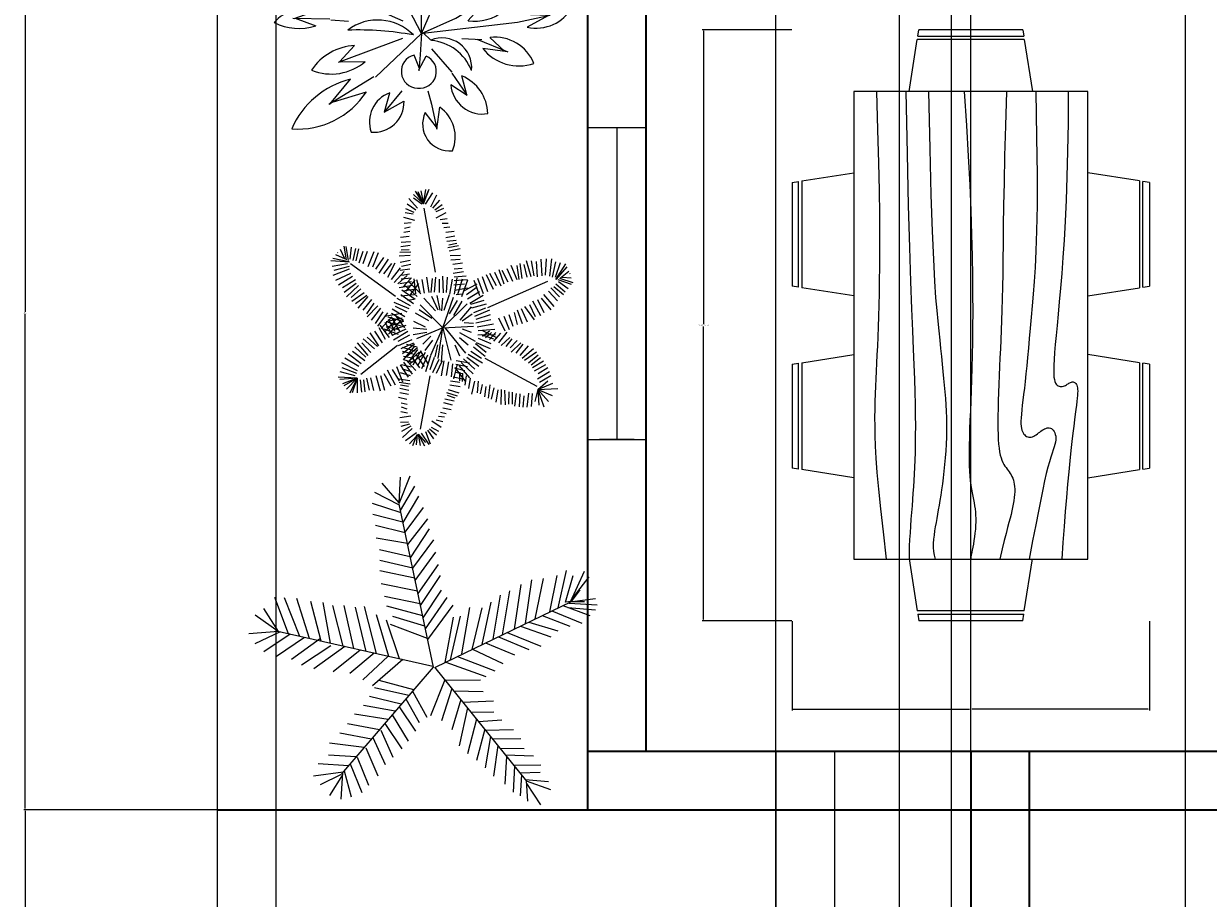
# Model space of a CAD drawing. Units: inches. Extents: x 450 to 1026, y 542 to 1190.
# Tile 5 of 11: x 450 to 632, y 804 to 939. Entities that reach past the tile are written whole.
import ezdxf

# ---------------------------------------------------------------- set-up
doc = ezdxf.new("R2010")
doc.units = ezdxf.units.IN
doc.header["$MEASUREMENT"] = 0
for name, color, linetype, lineweight in [('A-ANNO-DIMS', 2, 'Continuous', 18), ('A-FLOR', 8, 'Continuous', 25), ('A-FURN', 8, 'Continuous', 18), ('A-GLAZ', 4, 'Continuous', 18), ('A-WALL', 7, 'Continuous', 35), ('C-PROP', 7, 'Continuous', 25), ('L-PLNT', 3, 'Continuous', 13)]:
    doc.layers.add(name, color=color, linetype=linetype, lineweight=lineweight)
doc.styles.get("Standard").update_dxf_attribs({"font": 'arial.ttf'})
doc.dimstyles.get("Standard").update_dxf_attribs({"dimtxt": 0.18, "dimasz": 0.18, "dimexe": 0.18, "dimexo": 0.0625, "dimgap": 0.09, "dimtad": 0, "dimtih": 1, "dimtoh": 1, "dimdec": 4, "dimzin": 0, "dimdsep": 46, "dimtxsty": 'Standard', "dimcen": 0.09, "dimadec": 0, "dimazin": 0, "dimtfac": 1, "dimtdec": 4, "dimtofl": 0, "dimtmove": 0, "dimatfit": 3, "dimfxl": 1, "dimtolj": 1, "dimtzin": 0, "dimarcsym": 0})

# ---------------------------------------------------------------- blocks, each defined once
blk = doc.blocks.new('Dining Set - 36 x 72 in.')
for p, q in [((-22, 27.5), (-22.1562, 26.50042)), ((-22, 27.5), (-6, 27.5)), ((-5.8437, 26.49966), (-6, 27.5)), ((6, 27.5), (5.8438, 26.50042)), ((6, 27.5), (22, 27.5)), ((22.1563, 26.49966), (22, 27.5)), ((-22.2343, 26.00059), (-23.4847, 17.99762)), ((-22.2304, 26), (-5.7608, 26)), ((-5.8416, 26.5), (-22.1534, 26.5)), ((-4.5152, 17.99762), (-5.7655, 25.99926)), ((5.7657, 26.00059), (4.5153, 17.99762)), ((5.7696, 26), (22.2392, 26)), ((22.1584, 26.5), (5.8466, 26.5)), ((23.4848, 17.99762), (22.2345, 25.99926)), ((36, 18), (-36, 18)), ((-36, 18), (-36, -18)), ((36, -18), (36, 18)), ((-44.0006, 8.23428), (-35.9976, 9.48474)), ((44.0006, 8.23428), (35.9976, 9.48474)), ((-45.5, 8), (-44.5004, 8.15617)), ((-45.5, 8), (-45.5, -8)), ((-44.5, -8.15843), (-44.5, 8.15338)), ((-44, 8.23041), (-44, -8.23915)), ((44, 8.23041), (44, -8.23915)), ((44.5, -8.15843), (44.5, 8.15338)), ((45.5, 8), (44.5005, 8.15617)), ((45.5, 8), (45.5, -8)), ((-44.4997, -8.15631), (-45.5, -8)), ((-35.9976, -9.48476), (-43.9993, -8.2345)), ((35.9976, -9.48476), (43.9993, -8.2345)), ((44.4997, -8.15631), (45.5, -8)), ((-36, -18), (36, -18)), ((-22.2343, -26.0006), (-23.4847, -17.99762)), ((-4.5152, -17.99762), (-5.7655, -25.99928)), ((5.7657, -26.0006), (4.5153, -17.99762)), ((23.4848, -17.99762), (22.2345, -25.99928)), ((-22.2304, -26), (-5.7608, -26)), ((-22, -27.5), (-22.1562, -26.50044)), ((-5.8416, -26.5), (-22.1534, -26.5)), ((-5.8437, -26.49967), (-6, -27.5)), ((5.7696, -26), (22.2392, -26)), ((6, -27.5), (5.8438, -26.50044)), ((22.1584, -26.5), (5.8466, -26.5)), ((22.1563, -26.49967), (22, -27.5)), ((-22, -27.5), (-6, -27.5)), ((6, -27.5), (22, -27.5))]:
    blk.add_line(p, q)
for points in [[(-36, 15), (-31.1772, 14.97754), (-26.8079, 14.91406), (-22.8538, 14.81543), (-19.276, 14.6875), (-16.0362, 14.53613), (-13.0957, 14.36718), (-10.4159, 14.18652), (-7.9583, 14), (-5.6904, 13.81315), (-3.6035, 13.63021), (-1.6954, 13.45508), (0.0365, 13.29166), (1.5945, 13.14388), (2.9811, 13.01562), (4.1988, 12.9108), (5.25, 12.83333), (6.1393, 12.78613), (6.8802, 12.76823), (7.4883, 12.77767), (7.9792, 12.8125), (8.3685, 12.87077), (8.6719, 12.95052), (8.9049, 13.0498), (9.0833, 13.16666), (9.2205, 13.29899), (9.3216, 13.44401), (9.3895, 13.59879), (9.4271, 13.76041), (9.4373, 13.92594), (9.4232, 14.09245), (9.3875, 14.257), (9.3333, 14.41666), (9.2638, 14.56917), (9.1836, 14.71484), (9.0975, 14.85465), (9.0104, 14.98958), (8.9272, 15.1206), (8.8529, 15.2487), (8.7922, 15.37483), (8.75, 15.5), (8.7305, 15.62467), (8.7344, 15.74739), (8.7617, 15.86621), (8.8125, 15.97916), (8.8867, 16.08431), (8.9844, 16.17968), (9.1055, 16.26334), (9.25, 16.33333), (9.4189, 16.38802), (9.6172, 16.42708), (9.8506, 16.45052), (10.125, 16.45833), (10.4463, 16.45052), (10.8203, 16.42708), (11.2529, 16.38802), (11.75, 16.33333), (12.3184, 16.26318), (12.9694, 16.17838), (13.7151, 16.07991), (14.5677, 15.96875), (15.5395, 15.84586), (16.6426, 15.71224), (17.8893, 15.56884), (19.2917, 15.41666), (20.859, 15.25667), (22.5879, 15.08984), (24.4721, 14.91715), (26.5052, 14.73958), (28.6809, 14.5581), (30.9929, 14.3737), (33.4347, 14.18733), (36, 14)], [(-36, 10), (-28.9766, 10.14274), (-23.1725, 10.20442), (-18.4241, 10.19775), (-14.5677, 10.13541), (-11.4399, 10.03011), (-8.877, 9.89453), (-6.7154, 9.74137), (-4.7917, 9.58333), (-2.9698, 9.43082), (-1.2246, 9.28515), (0.4415, 9.14534), (2.026, 9.01041), (3.5266, 8.87939), (4.9408, 8.7513), (6.266, 8.62516), (7.5, 8.5), (8.6411, 8.37549), (9.6914, 8.2539), (10.6538, 8.13818), (11.5312, 8.03125), (12.3267, 7.93603), (13.043, 7.85547), (13.6831, 7.79248), (14.25, 7.75), (14.7471, 7.7303), (15.1797, 7.73307), (15.5537, 7.75732), (15.875, 7.80208), (16.1494, 7.86637), (16.3828, 7.94922), (16.5811, 8.04964), (16.75, 8.16666), (16.8944, 8.29915), (17.0143, 8.44531), (17.1089, 8.60319), (17.1771, 8.77083), (17.218, 8.94629), (17.2305, 9.1276), (17.2137, 9.31282), (17.1667, 9.5), (17.0895, 9.6875), (16.987, 9.875), (16.8649, 10.0625), (16.7292, 10.25), (16.5856, 10.4375), (16.4401, 10.625), (16.2985, 10.8125), (16.1667, 11), (16.05, 11.18733), (15.9518, 11.3737), (15.8752, 11.5581), (15.8229, 11.73958), (15.798, 11.91715), (15.8034, 12.08984), (15.842, 12.25667), (15.9167, 12.41666), (16.0295, 12.56836), (16.1784, 12.70833), (16.3605, 12.83268), (16.5729, 12.9375), (16.8127, 13.01888), (17.0768, 13.07291), (17.3625, 13.0957), (17.6667, 13.08333), (17.9894, 13.03312), (18.3418, 12.94726), (18.7382, 12.82918), (19.1927, 12.68229), (19.7195, 12.51001), (20.3327, 12.31575), (21.0465, 12.10294), (21.875, 11.875), (22.8357, 11.63354), (23.959, 11.37304), (25.2786, 11.08618), (26.8282, 10.76562), (28.6414, 10.40405), (30.752, 9.99414), (33.1936, 9.52856), (36, 9)], [(-36, 5.5), (-30.7157, 5.3348), (-26.069, 5.20963), (-21.9946, 5.11767), (-18.4271, 5.05208), (-15.3009, 5.00602), (-12.5508, 4.97265), (-10.1112, 4.94515), (-7.9167, 4.91666), (-5.909, 4.88167), (-4.0586, 4.83984), (-2.3429, 4.79215), (-0.7396, 4.73958), (0.7739, 4.6831), (2.22, 4.6237), (3.6213, 4.56233), (5, 4.5), (6.373, 4.43782), (7.7344, 4.3776), (9.0723, 4.32129), (10.375, 4.27083), (11.6309, 4.22819), (12.8281, 4.19531), (13.9551, 4.17415), (15, 4.16666), (15.954, 4.17448), (16.819, 4.19791), (17.6001, 4.23698), (18.3021, 4.29166), (18.9299, 4.36198), (19.4883, 4.44791), (19.9823, 4.54948), (20.4167, 4.66666), (20.7969, 4.79899), (21.1302, 4.94401), (21.4245, 5.09879), (21.6875, 5.26041), (21.9271, 5.42594), (22.1511, 5.59245), (22.3672, 5.757), (22.5834, 5.91666), (22.8065, 6.06868), (23.0404, 6.21093), (23.2879, 6.34147), (23.5521, 6.45833), (23.8358, 6.55957), (24.142, 6.64323), (24.4735, 6.70735), (24.8334, 6.75), (25.2235, 6.76969), (25.642, 6.76692), (26.0858, 6.74267), (26.5521, 6.69791), (27.0379, 6.63362), (27.5404, 6.55078), (28.0565, 6.45036), (28.5834, 6.33333), (29.1242, 6.19987), (29.7071, 6.04687), (30.3661, 5.87044), (31.1354, 5.66666), (32.0493, 5.43164), (33.142, 5.16146), (34.4475, 4.85221), (36, 4.5)], [(-36, -1), (-30.7915, -0.6591), (-26.0195, -0.38216), (-21.6519, -0.16284), (-17.6563, 0.00521), (-14.0005, 0.12833), (-10.6523, 0.21289), (-7.5796, 0.26522), (-4.75, 0.29166), (-2.134, 0.29793), (0.2878, 0.28711), (2.5317, 0.26163), (4.6146, 0.22396), (6.5529, 0.17651), (8.3633, 0.12174), (10.0623, 0.06209), (11.6667, 0), (13.1899, -0.06201), (14.6341, -0.1211), (15.9982, -0.17432), (17.2813, -0.21875), (18.4823, -0.25147), (19.6003, -0.26953), (20.6343, -0.27002), (21.5834, -0.25), (22.4481, -0.20768), (23.2357, -0.14584), (23.9549, -0.06836), (24.6146, 0.02083), (25.2235, 0.11784), (25.7904, 0.21875), (26.3241, 0.31966), (26.8334, 0.41666), (27.3265, 0.50618), (27.8099, 0.58593), (28.2894, 0.65397), (28.7709, 0.70833), (29.2601, 0.74707), (29.763, 0.76823), (30.2855, 0.76985), (30.8334, 0.75), (31.4088, 0.70784), (31.9994, 0.64713), (32.589, 0.57275), (33.1615, 0.48958), (33.7008, 0.4025), (34.1908, 0.3164), (34.6153, 0.23616), (34.9584, 0.16666), (35.2099, 0.11165), (35.3848, 0.07031), (35.504, 0.04069), (35.5886, 0.02083), (35.6594, 0.00879), (35.7377, 0.0026), (35.8442, 0.00032), (36, 0)], [(-36, -6.5), (-27.1843, -6.31267), (-20.084, -6.1263), (-14.469, -5.9419), (-10.1094, -5.76042), (-6.7752, -5.58285), (-4.2363, -5.41016), (-2.2629, -5.24333), (-0.625, -5.08334), (0.8708, -4.93099), (2.2715, -4.78646), (3.5872, -4.64974), (4.8281, -4.52084), (6.0046, -4.39974), (7.127, -4.28646), (8.2053, -4.18099), (9.25, -4.08334), (10.2705, -3.99382), (11.2734, -3.91407), (12.2647, -3.84603), (13.25, -3.79167), (14.2354, -3.75293), (15.2266, -3.73177), (16.2295, -3.73015), (17.25, -3.75), (18.2912, -3.79248), (19.3451, -3.85547), (20.4009, -3.93604), (21.4479, -4.03125), (22.4754, -4.13819), (23.4727, -4.25391), (24.4289, -4.37549), (25.3334, -4.5), (26.1785, -4.62492), (26.9694, -4.74935), (27.7145, -4.87281), (28.4219, -4.99479), (29.1, -5.11483), (29.7572, -5.23242), (30.4016, -5.34709), (31.0417, -5.45834), (31.6837, -5.56437), (32.3262, -5.65821), (32.9658, -5.73153), (33.599, -5.77604), (34.2224, -5.78345), (34.8327, -5.74545), (35.4264, -5.65373), (36, -5.5)], [(-36, -10), (-26.4022, -9.81299), (-18.4675, -9.62891), (-11.9839, -9.45069), (-6.7396, -9.28125), (-2.5226, -9.12354), (0.8789, -8.98047), (3.6769, -8.85498), (6.0833, -8.75), (8.2767, -8.66765), (10.3021, -8.60677), (12.1712, -8.56543), (13.8958, -8.54167), (15.4876, -8.53353), (16.9583, -8.53907), (18.3197, -8.55632), (19.5834, -8.58334), (20.7616, -8.61841), (21.8685, -8.66081), (22.9188, -8.71004), (23.9271, -8.76563), (24.9081, -8.82707), (25.8763, -8.89388), (26.8465, -8.96558), (27.8334, -9.04167), (28.8474, -9.12118), (29.8828, -9.20117), (30.93, -9.27824), (31.9792, -9.34896), (33.0205, -9.40991), (34.0443, -9.45768), (35.0407, -9.48885), (36, -9.5)], [(-36, -14.5), (-30.0881, -14.33513), (-25.0332, -14.21224), (-20.7312, -14.12647), (-17.0781, -14.07292), (-13.97, -14.04671), (-11.3027, -14.04297), (-8.9724, -14.05681), (-6.875, -14.08334), (-4.9224, -14.11833), (-3.0905, -14.16016), (-1.3709, -14.20785), (0.2448, -14.26042), (1.7647, -14.3169), (3.1973, -14.3763), (4.5507, -14.43767), (5.8333, -14.5), (7.0554, -14.5621), (8.235, -14.62175), (9.3922, -14.67652), (10.5469, -14.72396), (11.7192, -14.76164), (12.929, -14.78711), (14.1965, -14.79794), (15.5417, -14.79167), (16.9933, -14.76424), (18.6152, -14.70508), (20.4804, -14.60197), (22.6615, -14.44271), (25.2312, -14.21509), (28.2624, -13.9069), (31.8277, -13.50594), (36, -13)]]:
    blk.add_lwpolyline(points)
blk = doc.blocks.new('*U3')
for p, q in [((0, 100), (0, 0)), ((900, 100), (900, 0)), ((0, 50), (900, 50))]:
    blk.add_line(p, q)
blk = doc.blocks.new('z_83')
for p, q in [((-89.4, 429.3), (-60.3, 501.4)), ((-88.9, 430.3), (-133.6, 482.5)), ((-88.7, 431), (-85.1, 498.3)), ((-85.4, 410.6), (-47.4, 474.2)), ((-88.4, 424.7), (-153.2, 457.5)), ((-78.7, 379), (-37, 448.6)), ((-84.1, 404.4), (-159.4, 429.1)), ((1.5, -1.8), (-88.9, 427.1)), ((-73.4, 353.5), (-24.6, 418.7)), ((-78.9, 379.5), (-158.5, 400.3)), ((-66.6, 321.4), (-13.8, 388.7)), ((-72.9, 351.4), (-151.3, 371.2)), ((-59.2, 286.2), (-9.3, 362.5)), ((-67.1, 323.6), (-149.2, 337.4)), ((-53.4, 258.9), (2.3, 332.9)), ((-59.7, 288.6), (-140.8, 307.1)), ((-46.6, 226.6), (7.8, 301)), ((-53.4, 258.8), (-140.3, 279.1)), ((-47.8, 232), (-139.7, 251.7)), ((-39.3, 191.9), (14.8, 268.1)), ((329.4, 154.1), (351.1, 252.7)), ((361.7, 169.7), (398.6, 250.7)), ((-32.6, 160.2), (19.7, 239.3)), ((243.9, 112.8), (260.3, 228.4)), ((269.2, 125.1), (290.8, 231.4)), ((307.2, 143.4), (327.2, 239.5)), ((348.6, 168.9), (369.3, 239.7)), ((363.7, 174.3), (411.5, 235.7)), ((-40.5, 197.7), (-136.3, 217.6)), ((-25.7, 127.5), (22.6, 200.7)), ((158.7, 71.6), (177.8, 187.8)), ((183.3, 83.5), (202.6, 199.1)), ((214.3, 98.5), (232.2, 215.8)), ((364.9, 171.3), (387.8, 201.6)), ((-380.1, 85.7), (-416.6, 181.3)), ((-350.7, 79.1), (-390.7, 180.9)), ((-324.8, 73.3), (-358.6, 179)), ((-294.3, 66.4), (-321.3, 171.1)), ((-270.1, 60.9), (-288.7, 168.1)), ((-236.3, 53.3), (-263.7, 160.8)), ((-208.4, 47), (-233.9, 160.8)), ((-148.8, 33.6), (-179.9, 157.9)), ((-33.5, 164.5), (-127.9, 184.3)), ((-26.9, 133.2), (-121.3, 158.3)), ((-19.7, 98.7), (37.3, 181.5)), ((-13.8, 71.1), (53.1, 161.6)), ((6.4, -2), (364.9, 171.3)), ((129.5, 57.5), (153, 169.1)), ((341.7, 160.1), (412.5, 134)), ((364.9, 171.3), (348.6, 168.9)), ((358.4, 166.2), (432.2, 162.4)), ((364.9, 171.3), (398.4, 171.3)), ((366.2, 171.3), (427.8, 179)), ((-404.6, 89.8), (-467.8, 135)), ((-406.3, 91.7), (-445.1, 152.8)), ((-175.5, 39.6), (-203.6, 155.7)), ((-115.8, 26.1), (-148.6, 136.2)), ((-21.2, 106.1), (-105.8, 131.3)), ((31.8, 10.3), (54.2, 129.9)), ((46.5, 17.4), (72.6, 132.3)), ((76.4, 33.1), (97.4, 155.1)), ((103.3, 44.8), (129.8, 154.5)), ((287.8, 134), (360.5, 106.2)), ((313, 146.2), (391.8, 113.7)), ((355, 155.1), (428, 148.6)), ((-88.3, 19.9), (-122.5, 122)), ((-14.3, 73.3), (-111.5, 110.4)), ((230.1, 106.1), (310.3, 77.7)), ((252.3, 116.9), (328.3, 93.8)), ((-406.9, 91.5), (-484.5, 85.7)), ((-402.5, 90.8), (-468.8, 59.3)), ((-375.7, 84.8), (-444.9, 38.2)), ((-338.1, 76.3), (-411.7, 26.2)), ((0, 0), (-404.5, 91.3)), ((-296, 73.1), (-372.3, 18.3)), ((172.2, 78.2), (251.9, 44.7)), ((195.4, 89.4), (283.6, 53.4)), ((-268.9, 54.3), (-345.7, 3)), ((-231.6, 52.3), (-313.7, -6.1)), ((-191.4, 43.2), (-262.3, -14.6)), ((-154.8, 34.9), (-218.4, -18.5)), ((103.9, 45.2), (183.9, 7.7)), ((138.2, 61.7), (214.8, 30.4)), ((-117.9, 26.6), (-184.8, -35.7)), ((-79.7, 18), (-158.8, -51.2)), ((33.9, 11.3), (139.5, -27)), ((65, 26.4), (162.4, -12)), ((0.2, -1.8), (-240.5, -283.2)), ((4.4, -2), (246.2, -302.4)), ((-63.7, -76.5), (-154.1, -56)), ((-50.8, -61.4), (-141.8, -37.4)), ((31.2, -35.3), (-6.6, -130.5)), ((49.4, -58), (22.2, -143.5)), ((32.2, -36.5), (125.5, -35.3)), ((-83.6, -99.7), (-167.4, -79.2)), ((-71, -85), (-36.2, -147.6)), ((-54.2, -65.4), (-15.9, -133.4)), ((72.9, -87.1), (49.5, -167.3)), ((54.8, -64.7), (131.7, -66.4)), ((78.4, -94), (159, -90.5)), ((-99.2, -118), (-182.7, -102.7)), ((-89.2, -106.3), (-45.7, -170.7)), ((90.6, -109), (69, -209.5)), ((99.5, -120.1), (160.2, -120)), ((-141, -166.8), (-225.4, -151.2)), ((-118.1, -140.1), (-206.2, -126.1)), ((-127.1, -150.6), (-82.3, -217)), ((-107.6, -127.7), (-65.6, -196.7)), ((114.9, -139.3), (90.8, -230.4)), ((119.8, -145.4), (181.2, -140.7)), ((-162.1, -191.5), (-244.9, -176)), ((-136.8, -167.6), (-105.8, -239.3)), ((136.1, -165.5), (114.9, -247.8)), ((137.8, -167.7), (211.7, -166.4)), ((151.5, -184.7), (137.8, -267.3)), ((-180.8, -213.4), (-272.2, -202.2)), ((-176.3, -214), (-145.2, -287.8)), ((-158.7, -187.5), (-125.7, -258.4)), ((156.6, -191), (231.1, -189.4)), ((170.5, -208.3), (159, -289)), ((176.4, -215.7), (240.4, -216.2)), ((-202.3, -238.5), (-275.4, -233.4)), ((-199.9, -238.7), (-169.5, -312.8)), ((193.8, -237.2), (189.2, -310.2)), ((190.5, -233.2), (264.8, -235.3)), ((-236.3, -278.2), (-314.1, -289)), ((-222.2, -261.8), (-302.1, -256.4)), ((-238.2, -280.5), (-242.6, -349.9)), ((-233.5, -275), (-215.7, -343.6)), ((-218, -256.9), (-187.5, -331.7)), ((214.3, -262.7), (210.8, -331.5)), ((211.8, -259.6), (283.6, -259.4)), ((228.7, -280.6), (282.1, -278.9)), ((-241.3, -284.2), (-297, -312)), ((-238.5, -285.9), (-272.6, -339.8)), ((232.7, -285.6), (229.4, -340.8)), ((242.3, -297.5), (304.2, -303.2)), ((245.3, -301.2), (309, -324)), ((245.6, -301.6), (248.9, -354.6)), ((246.1, -308.6), (283.2, -364.8))]:
    blk.add_line(p, q)
blk = doc.blocks.new('z_86')
for p, q in [((-83.5, 478), (-122.3, 513.6)), ((-83.5, 478), (-114.5, 526.5)), ((-83.5, 478), (-106.5, 517.8)), ((-105.6, 525.2), (-83.5, 478)), ((-94.4, 527.5), (-83.5, 478)), ((-83.5, 478), (-61.2, 534.1)), ((-83.5, 478), (-75.1, 533.5)), ((-83.5, 478), (-65.1, 526.2)), ((-76.2, 477.3), (-47.6, 520.2)), ((-55.2, 467.1), (-32.4, 512)), ((-118.8, 445.3), (-151.4, 458.3)), ((-112.8, 453.1), (-146, 476.4)), ((-106.9, 460.9), (-139.8, 499)), ((-89.5, 477.3), (-121.9, 499.8)), ((-36.9, 215.2), (-81.5, 462)), ((-47.6, 461), (-21, 491.6)), ((-40, 454.9), (-11.4, 475.3)), ((-34.3, 448.8), (-5.7, 461)), ((-117, 414.2), (-158.9, 425)), ((-122.8, 438), (-153.5, 443.1)), ((-34.3, 424.3), (3.8, 444.7)), ((-19.1, 418.2), (7.6, 422.3)), ((-135.9, 371.8), (-158.6, 368.3)), ((-130.3, 404.7), (-157.2, 402.3)), ((-134.3, 389), (-156.5, 383.5)), ((-11.4, 403.9), (11.4, 403.9)), ((-5.7, 387.6), (17.1, 389.6)), ((1.9, 369.2), (34.3, 373.3)), ((-138.9, 352.1), (-171.3, 348.3)), ((-134, 332.3), (-168.8, 330.1)), ((1.9, 348.8), (36.2, 354.9)), ((5.7, 334.5), (41.9, 338.6)), ((13.3, 320.3), (43.8, 326.4)), ((-382.4, 265.8), (-420.1, 282.2)), ((-412.2, 291.3), (-413.8, 289.4)), ((-387.3, 269.9), (-402.1, 302.2)), ((-379.4, 263.2), (-388.4, 316.1)), ((-371.9, 259.8), (-379.8, 313.8)), ((-365.6, 265.3), (-360, 311.4)), ((-353.9, 260.7), (-343.8, 307)), ((-341.4, 258.8), (-331.3, 305.1)), ((-330.6, 251.5), (-315.1, 296.4)), ((-315.3, 248.9), (-298.9, 296.4)), ((-295.6, 237.8), (-272.9, 295.1)), ((-278.5, 236), (-256.7, 290.7)), ((-134.8, 279.6), (-177.4, 277.5)), ((-132.2, 292.8), (-174.8, 290.8)), ((-134.3, 317.5), (-170.4, 312.8)), ((-138.3, 301.8), (-169.4, 300.5)), ((9.5, 310), (51.4, 318.2)), ((15.2, 297.8), (57.1, 306)), ((19, 279.5), (59, 281.5)), ((-368.1, 253.4), (-438.9, 258.6)), ((-374.7, 247.6), (-434, 237.7)), ((-370, 255.1), (-431.7, 268)), ((-369.3, 237.5), (-427.8, 221.6)), ((-190.5, 122.3), (-363.9, 247)), ((-266.9, 227.1), (-235.2, 271.9)), ((-254.3, 212.2), (-218.1, 265.9)), ((-236.4, 208.8), (-204.7, 249.3)), ((-220.3, 195.8), (-192.1, 251.6)), ((-206.8, 187.8), (-172.4, 231.9)), ((-134.1, 260.9), (-173.4, 253.3)), ((-132, 244.6), (-167.7, 237.9)), ((20.9, 263.1), (57.1, 265.2)), ((28.5, 246.8), (66.6, 250.9)), ((34.3, 228.4), (64.7, 230.5)), ((258.9, 179.5), (238, 228.4)), ((276.1, 185.6), (253.2, 240.7)), ((274.2, 240.7), (281.8, 187.7)), ((295.1, 191.7), (287.5, 248.9)), ((314.1, 195.8), (302.7, 244.8)), ((329.4, 197.9), (312.2, 259.1)), ((340.8, 201.9), (331.3, 259.1)), ((354.1, 197.9), (350.3, 257)), ((371.3, 201.9), (367.5, 265.2)), ((384.6, 204), (388.4, 267.2)), ((401.7, 199.9), (409.4, 267.2)), ((411.2, 195.8), (424.6, 255)), ((422.7, 195.8), (441.7, 252.9)), ((424.7, 187.2), (462.5, 247.4)), ((427.1, 188.2), (467.4, 236.7)), ((-368.5, 227.2), (-431.5, 202.4)), ((-364.1, 210.1), (-421.7, 183.9)), ((-356, 199.3), (-410.1, 166.3)), ((-344.4, 186.1), (-394.9, 155)), ((-196.1, 176.3), (-158.1, 217.9)), ((-181.7, 171), (-145.6, 203)), ((-135.5, 226.9), (-173.5, 221.8)), ((-129.1, 192.8), (-169.4, 189.2)), ((-136.7, 207.7), (-166.7, 202.4)), ((-164.7, 156.3), (-132.2, 190.7)), ((-150.4, 142.3), (-115.1, 184.7)), ((-113.5, 132.6), (-119.3, 190.6)), ((-96.8, 137.1), (-108.7, 186)), ((-79.7, 135.1), (-88.7, 187.5)), ((-61.5, 137.1), (-71, 196)), ((-50.7, 191.1), (-55.5, 137.7)), ((-41.6, 138.6), (-35.8, 196)), ((-22.2, 138.2), (-21.9, 188.5)), ((-6.8, 136.7), (-9.4, 200.2)), ((5.2, 138), (9.1, 195.8)), ((17.2, 130.9), (27.2, 189.4)), ((30.5, 212.1), (70.4, 218.3)), ((34.3, 197.9), (80, 201.9)), ((34.3, 183.6), (85.7, 187.7)), ((34.8, 130.9), (45.8, 193.4)), ((48.3, 129.9), (66.6, 190.5)), ((64, 121.9), (87, 185.6)), ((133.3, 124.4), (110.4, 183.6)), ((146.6, 132.6), (125.6, 191.7)), ((163.7, 140.7), (142.8, 197.9)), ((184.7, 148.9), (158, 206)), ((196.1, 163.2), (171.3, 210.1)), ((188.5, 216.2), (213.2, 163.2)), ((226.6, 169.3), (207.5, 224.4)), ((241.8, 177.5), (218.9, 222.4)), ((432.2, 187.7), (483.6, 169.3)), ((438.7, 192.7), (489.7, 175.9)), ((442.4, 194.2), (474.5, 219.7)), ((448.3, 196.5), (483.8, 194.5)), ((478.9, 208.5), (478, 210.8)), ((-341.8, 172.4), (-387.8, 137.2)), ((-332.8, 164.2), (-378.9, 120.4)), ((-323.9, 151.7), (-361.8, 118.7)), ((-311.3, 136.8), (-358.3, 103.3)), ((-125.9, 164.1), (-176.8, 155.8)), ((-129.4, 178), (-174.7, 171)), ((-114.9, 110.1), (-166.7, 146.7)), ((-120.2, 148.7), (-161.8, 142.7)), ((-108.2, 121.8), (-155.1, 164.3)), ((-94.3, 132.6), (-142, 180.7)), ((-135.2, 126.7), (-101.7, 172.4)), ((32.3, 167.2), (74.2, 171.3)), ((36.2, 146.9), (85.7, 155)), ((70.9, 144), (122.8, 170.4)), ((81, 130), (122.3, 158.8)), ((85.4, 113.4), (131, 140.8)), ((163.8, 79.8), (394.1, 180.6)), ((396, 142.8), (430.3, 106.1)), ((405.5, 155), (437.9, 120.3)), ((417, 161.2), (453.2, 130.5)), ((424.6, 171.3), (460.8, 140.7)), ((434.1, 179.5), (472.2, 153)), ((-344.8, 95.3), (-301.5, 126.9)), ((-297, 122.8), (-335, 76.8)), ((-283.6, 110.5), (-317, 69.1)), ((-273.8, 96.3), (-302.7, 55.1)), ((-138, 74.9), (-196.4, 99.8)), ((-134, 86.3), (-184.5, 114.7)), ((-122.5, 94.2), (-171, 128.2)), ((-119, 128), (-169, 124.1)), ((-120.6, 110.8), (-145.2, 106.9)), ((-38.1, 67.3), (-81.9, 116.3)), ((-26.7, 69.3), (-51.4, 122.4)), ((-19.1, 69.3), (-30.5, 126.5)), ((-13.3, 67.3), (-9.5, 116.3)), ((-9.5, 2), (31.9, 119.3)), ((-9.5, 2), (83.8, 94.2)), ((-3.8, 69.5), (16, 129.9)), ((16.7, 55.7), (46.5, 106.9)), ((33.2, 49.6), (65.3, 104.2)), ((41.9, 130.5), (66.6, 132.6)), ((93.8, 97.2), (145.2, 127.4)), ((148.1, 106.6), (96.6, 91.8)), ((102.5, 79.2), (158, 94.6)), ((323.7, 91.8), (344.6, 44.9)), ((335.1, 106.1), (365.5, 48.9)), ((354.1, 110.1), (378.9, 61.2)), ((367.5, 116.3), (405.5, 71.4)), ((377, 130.5), (417, 83.6)), ((-259.4, 86.7), (-299.2, 44.1)), ((-283.1, 31.1), (-247.8, 77.8)), ((-239.8, 62.7), (-269.6, 18.8)), ((-221.8, 59.2), (-259.8, 8.9)), ((-166.3, 56.4), (-233.1, 45)), ((-206, 58.7), (-159.8, 31.4)), ((-154.7, 44.3), (-204, 74.1)), ((-155.8, 1.7), (-191.5, 50.9)), ((-145.9, 61.7), (-191.3, 83.5)), ((-63.5, 29.2), (-114, 57.6)), ((-52, 37.1), (-100.5, 71.1)), ((-9.5, 2), (-96.2, 89.6)), ((57.4, 30.9), (101.2, 82.5)), ((64.7, 28.6), (102.8, 55.1)), ((109.1, 60.9), (156.1, 78.9)), ((113.3, 46.1), (171.5, 71.5)), ((118.9, 35.3), (174.1, 52.6)), ((224.7, 46.9), (245.6, -4.1)), ((243.7, 53), (258.9, 8.1)), ((264.6, 61.2), (276.1, 14.3)), ((276.1, 71.4), (295.1, 18.4)), ((291.3, 75.5), (314.1, 24.4)), ((304.6, 83.6), (340.8, 32.6)), ((-229.7, -42.7), (-254.3, 1.3)), ((-214.5, -34.6), (-249.6, 11.9)), ((-204.8, 44.6), (-245.5, -0.7)), ((-232.2, 23.2), (-202, -27)), ((-189.6, 33.2), (-232, -13)), ((-165.5, 38.8), (-227.2, 24.8)), ((-176.9, -6.2), (-226.2, 4.1)), ((-159.8, 26.6), (-219.4, 5.3)), ((-161.8, 25.7), (-219.1, 42.3)), ((-167.8, 8.5), (-219.1, 22.8)), ((-176.1, 25.3), (-217.7, -22.6)), ((-192.4, -12.7), (-217.6, 34)), ((-174.2, -11.2), (-206.8, 42.8)), ((-151.1, 11.3), (-206.8, -8.9)), ((-70.4, -4.1), (-123.8, 0)), ((-75.4, 4.6), (-120.8, 26.4)), ((-9.5, 2), (-110.4, -40.8)), ((-55.6, -103.4), (-9.5, 2)), ((-26.9, -115.3), (-9.5, 2)), ((-9.5, 2), (108.5, 8.1)), ((-9.5, 0), (20.9, -122.4)), ((0, 0), (78, -95.9)), ((72.4, 22.4), (108.5, 20.4)), ((116.7, 21.6), (174.7, 33.4)), ((123, 5.1), (185.2, 17.6)), ((203.7, 40.8), (228.5, -10.2)), ((-271.3, -79), (-314.5, -40.9)), ((-300.3, -34.4), (-260.5, -70.2)), ((-255.6, -66.7), (-288.6, -17)), ((-241, -55.8), (-270, -11.1)), ((-180.1, -23.2), (-234.9, -3.5)), ((-151.3, -2.6), (-203.4, -27.7)), ((-144.2, -12.5), (-198.1, -46)), ((-137.9, -26.5), (-181.8, -51.2)), ((-128.7, -43.7), (-181.4, -66.9)), ((-70.4, -16.3), (-123.8, -24.5)), ((-55.2, -30.6), (-85.7, -61.2)), ((-49.5, -44.9), (-78.1, -85.7)), ((55.2, -16.3), (114.2, -49)), ((55.2, -34.7), (87.6, -63.3)), ((64.7, -2.1), (99, -14.3)), ((125.2, -25.3), (192.9, -23.6)), ((126.3, -37.5), (175.2, -58.4)), ((126.9, -7.8), (190, -2.9)), ((137.2, -24.2), (184.8, -40.9)), ((142.6, -7.8), (194.4, -34.4)), ((142.8, -30.6), (169.5, -10.2)), ((154.2, -36.8), (177.1, -16.3)), ((169.5, -42.8), (194.2, -16.3)), ((186.6, -49), (213.2, -18.4)), ((205.6, -55.1), (238, -14.3)), ((215.1, -65.3), (247.5, -34.7)), ((234.2, -69.4), (257, -40.8)), ((-309.3, -124.6), (-356.3, -88.5)), ((-305.2, -111.3), (-347.4, -71.6)), ((-295.5, -104.1), (-336.7, -55.7)), ((-183, -66.2), (-324.2, -177.7)), ((-285.3, -92.6), (-319.6, -55.8)), ((-169.9, -77.5), (-121.1, -55.3)), ((-115, -87.4), (-164.7, -73.8)), ((-119.8, -100.8), (-164.2, -89.1)), ((-117.5, -60.2), (-164, -97.6)), ((-118.6, -68.3), (-161.5, -120.7)), ((-107.6, -72.7), (-148.4, -62.3)), ((-106.9, -75), (-148, -108.8)), ((-106.4, -81), (-143.8, -132.1)), ((-100.1, -90.9), (-136.8, -125.4)), ((-94.1, -86.5), (-125.1, -141.7)), ((-95, -87.2), (-66.5, -136.2)), ((-39.1, -109.5), (-28.6, -63.3)), ((-15, -128.2), (-9.5, -63.3)), ((36.2, -63.3), (55.2, -106.1)), ((97.6, -87.5), (139.7, -115)), ((108.5, -71.4), (153.5, -107.4)), ((157.5, -92.3), (115.4, -59.2)), ((118.1, -53.8), (172.7, -77.8)), ((249.4, -75.5), (276.1, -47)), ((253.2, -91.8), (289.4, -55.1)), ((272.2, -95.9), (298.9, -61.2)), ((287.5, -104.1), (319.9, -67.3)), ((295.1, -114.2), (338.9, -77.5)), ((304.6, -122.4), (350.3, -89.8)), ((-337.4, -163), (-397.6, -131.9)), ((-331.3, -146.5), (-385.9, -114.5)), ((-322.2, -136.6), (-372.6, -98.2)), ((-121.1, -115.5), (-160.8, -107.7)), ((-160.7, -130.3), (-127.3, -175.6)), ((-130.2, -129.6), (-159.6, -121.2)), ((-145.9, -126.4), (-113.3, -162.1)), ((-88, -103.2), (-135.6, -136.9)), ((-127.4, -113.6), (-98.7, -151.2)), ((-111.8, -101.2), (-81.1, -147)), ((-77.5, -92.3), (-106.3, -144.1)), ((-68.5, -102.9), (-91.4, -156.1)), ((-56.7, -105.7), (-75.4, -166.5)), ((-42.8, -112.2), (-59.7, -159.6)), ((-24.5, -119.1), (-49, -171.2)), ((-33.4, -171.6), (-11.1, -122.9)), ((-5.2, -124.2), (-15.8, -182.9)), ((12.5, -128.4), (3.6, -180.9)), ((28, -135.9), (23, -186.1)), ((42.3, -123.5), (93, -132.9)), ((60.6, -131.4), (107, -174.5)), ((70.1, -116.6), (113.7, -156.7)), ((82.6, -110.3), (128.9, -145)), ((88, -99.5), (142.7, -131.9)), ((151.4, -114), (352, -222.7)), ((319.9, -132.6), (356.1, -102)), ((329.4, -140.8), (365.5, -112.2)), ((335.1, -151), (377, -124.4)), ((-345.7, -182.7), (-403.8, -166.7)), ((-339.4, -173.2), (-395.9, -151.3)), ((-266.1, -181.1), (-249.4, -240.5)), ((-248.9, -181.2), (-232.8, -237.8)), ((-236.4, -173.5), (-209.5, -221.3)), ((-222.4, -160), (-191.9, -217.1)), ((-204.2, -158.4), (-176.9, -202)), ((-186.8, -147.2), (-164.6, -205.6)), ((-172.6, -140.6), (-143, -188)), ((-133.2, -182.8), (-171.5, -171.1)), ((-131.1, -148.8), (-168.3, -139.7)), ((-129.5, -166.7), (-164.2, -156.4)), ((45.2, -137.3), (31.5, -193.9)), ((35.5, -151.5), (74.7, -161.8)), ((37.1, -150.9), (78.1, -204.9)), ((37.6, -168.1), (67.7, -173.3)), ((40.8, -137.7), (85.8, -146.5)), ((52.3, -142.1), (93.3, -190.4)), ((54.3, -168.6), (55, -202.2)), ((66.2, -173.7), (64.5, -204.3)), ((80.5, -181.8), (75.2, -217.7)), ((342.7, -163.2), (386.5, -138.7)), ((354.1, -193.8), (399.8, -165.3)), ((356.1, -173.4), (394.1, -151)), ((361.7, -206.1), (405.5, -181.6)), ((-338.1, -191.4), (-410.8, -187.1)), ((-338.1, -191.4), (-404.6, -197.1)), ((-338.1, -191.4), (-394.5, -212.5)), ((-338.1, -191.4), (-389, -220.3)), ((-338.1, -191.4), (-378.7, -234.2)), ((-338.1, -191.4), (-366.5, -249.5)), ((-338.1, -191.4), (-357.7, -248.1)), ((-338.1, -191.4), (-337.7, -247.7)), ((-326.5, -197.9), (-321.2, -245)), ((-313.8, -197.3), (-308.5, -244.4)), ((-302.3, -191.2), (-291.5, -237.4)), ((-286.8, -190.1), (-275.4, -239)), ((-135.9, -201.3), (-178, -194.7)), ((-134.7, -214.7), (-176.8, -208.2)), ((-141.7, -223), (-172.4, -218.5)), ((-59.2, -183), (-96.3, -387.3)), ((17.1, -217.3), (56.7, -223.5)), ((20.7, -201.2), (56.5, -207.1)), ((30, -185.8), (67.5, -193.9)), ((96, -191.4), (88.7, -231.3)), ((112.6, -202.4), (100.9, -253.2)), ((126.6, -203.5), (122.8, -247.9)), ((141.6, -215.8), (133.6, -251.5)), ((155.9, -223.9), (150.3, -262.6)), ((171, -216.7), (164.9, -267.9)), ((355.4, -234.4), (394.1, -202)), ((355.4, -234.4), (413.2, -210.1)), ((-147.6, -273), (-179.4, -265.8)), ((-140.6, -253.8), (-175, -247.9)), ((-139.4, -239.1), (-174.8, -230.6)), ((-1.9, -270.6), (33.7, -278.5)), ((4.5, -246.7), (45.3, -259.2)), ((7.2, -257.2), (36.8, -266.5)), ((11.4, -235.1), (52.2, -247.6)), ((186.1, -229), (175.7, -271.5)), ((202, -235.8), (193.5, -284.1)), ((214.7, -235.4), (213.3, -292.5)), ((227, -237.7), (230.1, -293.8)), ((244.5, -243.3), (243.2, -290.7)), ((256.8, -245.6), (257.1, -291.7)), ((272.4, -249.9), (266.2, -299.1)), ((286.7, -251.6), (283.2, -301.6)), ((301.6, -259.3), (297.6, -303.3)), ((319.3, -248.8), (312.9, -302.4)), ((333.6, -250.5), (330.1, -300.5)), ((355.4, -234.4), (343.7, -281.5)), ((354.7, -235.1), (410.6, -257.7)), ((355.4, -234.4), (432.2, -230.9)), ((355.4, -234.4), (359.2, -295.3)), ((355.4, -234.4), (378.3, -301.1)), ((355.4, -234.4), (395.7, -281.2)), ((-146.7, -292.8), (-168.8, -287)), ((-146.8, -310.2), (-168.3, -302.4)), ((-9.3, -304.7), (22.5, -312.2)), ((-7.2, -284.4), (26.3, -294.1)), ((-132.2, -337.1), (-175, -343.3)), ((-140.6, -360.1), (-171.6, -361.9)), ((-144.5, -326.2), (-171, -321)), ((-51.1, -355.7), (-15.3, -380)), ((-35.3, -351.3), (-9.2, -358.1)), ((-26.2, -337.8), (-3.5, -340.2)), ((-18.8, -322.2), (3.7, -326.6)), ((-137.3, -367.8), (-171.1, -377.3)), ((-132.2, -376.2), (-167.6, -395.9)), ((-127.1, -384.5), (-163.8, -418.9)), ((-110.9, -401.2), (-152.3, -431.8)), ((-124.9, -449.3), (-107.4, -408)), ((-107.4, -408), (-111.5, -447.2)), ((-104.4, -407), (-96.1, -449.6)), ((-104.4, -407), (-79.8, -451)), ((-104.4, -407), (-75.5, -437.8)), ((-92.8, -402.8), (-63.3, -445.5)), ((-76.4, -396.1), (-58.3, -443.2)), ((-68.2, -390.9), (-44.9, -424.1)), ((-59.9, -385.6), (-33.7, -408.9)), ((-53.6, -380.1), (-26.5, -395.3)), ((-110.9, -413.5), (-137.9, -443.4))]:
    blk.add_line(p, q)
blk = doc.blocks.new('z_109')
for p, q in [((-93.8, 293.8), (-121.7, 396.4)), ((-120.7, 392.8), (-119, 324)), ((-120.3, 377.4), (-82.1, 322.4)), ((-4.7, 350.4), (-41.8, 295.2)), ((-14.4, 233.6), (-4.7, 350.4)), ((-4.7, 350.4), (24.2, 283.6)), ((-85.3, 244.1), (-94.4, 292.7)), ((65, 208.9), (149.6, 306.7)), ((149.6, 306.7), (68.1, 272.4)), ((129.3, 216), (149.6, 306.7)), ((149.6, 306.7), (129.3, 216)), ((-19.6, 10.5), (-18, 230)), ((-253.8, 128), (-391.6, 201.8)), ((-391.5, 201.8), (-278.3, 190.4)), ((-389.8, 201.6), (-326.7, 125.3)), ((-60.9, 91.7), (-127.6, 186)), ((-126.1, 183.9), (-59.8, 124.6)), ((-120.3, 175.7), (-91.5, 97.7)), ((-19.6, 10.5), (65, 204.6)), ((65, 204.6), (65, 204.6)), ((216.8, 135.4), (101.3, 104.7)), ((101.8, 63.8), (216.8, 135.4)), ((216.8, 135.4), (144.5, 54.6)), ((-467.5, 62.9), (-391.6, 89.6)), ((-83.6, 53.9), (-246.4, 124.8)), ((-19.6, 10.5), (-60.9, 91.7)), ((-342, 60.3), (-471.9, 63)), ((-463.4, 64.3), (-391.5, 36.9)), ((-275.7, 53), (-338.5, 56.9)), ((-19.6, 10.5), (101.8, 63.8)), ((-14.3, 11.4), (319, 50.5)), ((319, 50.5), (433.6, 75.1)), ((428.9, 74.1), (332.5, 76.8)), ((428.1, 74.1), (353.4, 32.3)), ((-19.6, 10.5), (-181.1, -143.2)), ((-19.6, 10.5), (-24.2, -64.6)), ((-19.6, 10.5), (-14.3, 11.4)), ((-14.3, 11.4), (-13.4, 12.7)), ((-13.4, 12.7), (13.4, -12.7)), ((-177.8, -41.4), (-312.5, -91.6)), ((-308.1, -89.9), (-254.4, -32.6)), ((-86.1, -7.9), (-177.8, -41.4)), ((122.5, -7.9), (193.1, -11)), ((176.2, -10.2), (284.5, -54.4)), ((272.8, -52.5), (222, -4.2)), ((-25.6, -113), (-45, -65.8)), ((-24.2, -64.6), (-28.2, -121)), ((-27.9, -117.3), (-2.3, -69.4)), ((15.9, -43.2), (88.2, -126.5)), ((283.1, -53.8), (196.2, -42.2)), ((-305.8, -89.1), (-217, -88.2)), ((-186.9, -142.9), (-344.9, -240)), ((-342.2, -238.3), (-268.6, -151.1)), ((87.3, -129.3), (139.6, -204.2)), ((140.4, -205.5), (123.1, -139.2)), ((-328.5, -229.9), (-213.2, -194.7)), ((-88.6, -191.8), (-150.4, -266.6)), ((-149.9, -266), (-130.8, -198.8)), ((3.5, -191.8), (15.9, -238.1)), ((141.1, -208), (83.6, -170.3)), ((-150.6, -266.9), (-80.7, -228.2)), ((15.9, -238.1), (35.2, -326.4)), ((35.2, -326.5), (45.1, -249.3)), ((33.8, -320.1), (-6.3, -268.4))]:
    blk.add_line(p, q)
for centre, radius, start, end in [((262.2, 393.4), 319.4, 140.563, 197.8988), ((-221.5, 433.3), 287.6, 328.6458, 34.5329), ((84.2, 468), 249.1, 170.3029, 215.3262), ((-234.9, 368.4), 159.6, 343.2534, 62.5239), ((255.6, 231.5), 191.8, 77.7318, 167.6805), ((55.5, 446.9), 242.5, 287.7269, 353.3689), ((-464.4, 59.2), 227.7, 35.1725, 122.5976), ((-304.3, 504.2), 379.6, 221.8384, 266.6027), ((-20.9, 238.7), 157.6, 161.4501, 243.415), ((-251.5, 114.8), 192, 2.9136, 65.0019), ((246.7, 85.9), 146.6, 55.2824, 172.6291), ((166.6, 217.1), 164, 262.2896, 356.2544), ((434.4, 8.1), 122.9, 51.1111, 145.9654), ((-434.4, -39.4), 135.9, 71.6414, 139.5892), ((384.1, 175.1), 146, 257.8549, 330.7421), ((-450, 225.2), 197.1, 243.5199, 287.2599), ((-172.9, -117.6), 175.2, 44.3837, 127.1057), ((-243.2, -1062.9), 1085.6, 79.6239, 91.8656), ((-246.3, -222.4), 190, 92.4489, 147.0817), ((52.6, -110.1), 105, 354.7987, 111.9005), ((1.6, -181.5), 167.4, 21.6922, 85.2277), ((240.6, -148.9), 145.9, 21.4559, 97.3107), ((-31.3, -123), 58.9, 103.4106, 268.148), ((-25.7, -123.5), 58.9, 262.5922, 66.6581), ((324.6, 60.3), 164.3, 218.6232, 288.4099), ((-336.9, 52.1), 184.6, 248.0932, 310.529), ((-198.2, -444.5), 301.7, 103.499, 156.8265), ((66, -275.9), 148.2, 1.4924, 67.3596), ((-454.6, -39.5), 287, 265.8156, 327.2626), ((-93.8, -301), 108.7, 109.8936, 199.3062), ((196.5, -160), 113.4, 185.1842, 278.9266), ((-186.1, -231.9), 105.5, 264.4232, 2.0221), ((-27.8, -353.9), 127.5, 337.3115, 55.0978), ((80, -308.4), 95.1, 155.1092, 275.9038)]:
    blk.add_arc(centre, radius, start, end)
blk = doc.blocks.new('WIN-FRAME-48IN')
for p, q in [((9, 48), (0, 48)), ((9, 0), (9, 48)), ((0, 0), (9, 0))]:
    blk.add_line(p, q)
blk = doc.blocks.new('*D29')
at = {"layer": 'A-ANNO-DIMS', "color": 0, "lineweight": -2, "transparency": 16777216}
for p, q in [((568.09, 938.05), (554.32, 938.05)), ((554.5, 937.87), (554.5, 892.73)), ((554.5, 847.23), (554.5, 892.36)), ((568.09, 847.05), (554.32, 847.05))]:
    blk.add_line(p, q, dxfattribs=at)
at = {"layer": 'A-ANNO-DIMS', "color": 0, "transparency": 16777216}
for points in [[(554.47, 937.87), (554.53, 937.87), (554.5, 938.05)], [(554.47, 847.23), (554.53, 847.23), (554.5, 847.05)]]:
    blk.add_solid(points, dxfattribs=at)
at = {"layer": 'Defpoints', "color": 0, "transparency": 16777216}
for p in [(568.15, 938.05), (554.5, 847.05), (568.15, 847.05)]:
    blk.add_point(p, dxfattribs=at)
at = {"layer": 'A-ANNO-DIMS', "color": 0, "transparency": 16777216, "insert": (554.5, 892.55), "char_height": 0.18, "attachment_point": 5}
blk.add_mtext('\\A1;DINING SET 91', dxfattribs=at)
blk = doc.blocks.new('*D30')
at = {"layer": 'A-ANNO-DIMS', "color": 0, "lineweight": -2, "transparency": 16777216}
for p, q in [((568.15, 846.99), (568.15, 833.22)), ((623.15, 846.99), (623.15, 833.22)), ((568.33, 833.4), (595.43, 833.4)), ((622.97, 833.4), (595.87, 833.4))]:
    blk.add_line(p, q, dxfattribs=at)
at = {"layer": 'A-ANNO-DIMS', "color": 0, "transparency": 16777216}
for points in [[(568.33, 833.43), (568.33, 833.37), (568.15, 833.4)], [(622.97, 833.43), (622.97, 833.37), (623.15, 833.4)]]:
    blk.add_solid(points, dxfattribs=at)
at = {"layer": 'Defpoints', "color": 0, "transparency": 16777216}
for p in [(568.15, 847.05), (623.15, 847.05), (623.15, 833.4)]:
    blk.add_point(p, dxfattribs=at)
at = {"layer": 'A-ANNO-DIMS', "color": 0, "transparency": 16777216, "insert": (595.65, 833.4), "char_height": 0.18, "attachment_point": 5}
blk.add_mtext('\\A1;55', dxfattribs=at)
blk = doc.blocks.new('*D52')
at = {"layer": 'A-ANNO-DIMS', "color": 0, "lineweight": -2, "transparency": 16777216}
for p, q in [((479.59, 970.94), (449.87, 970.94)), ((450.05, 970.76), (450.05, 894.62)), ((450.05, 818.12), (450.05, 894.26)), ((479.59, 817.94), (449.87, 817.94))]:
    blk.add_line(p, q, dxfattribs=at)
at = {"layer": 'A-ANNO-DIMS', "color": 0, "transparency": 16777216}
for points in [[(450.02, 970.76), (450.08, 970.76), (450.05, 970.94)], [(450.02, 818.12), (450.08, 818.12), (450.05, 817.94)]]:
    blk.add_solid(points, dxfattribs=at)
at = {"layer": 'Defpoints', "color": 0, "transparency": 16777216}
for p in [(479.65, 970.94), (450.05, 817.94), (479.65, 817.94)]:
    blk.add_point(p, dxfattribs=at)
at = {"layer": 'A-ANNO-DIMS', "color": 0, "transparency": 16777216, "insert": (450.05, 894.44), "char_height": 0.18, "attachment_point": 5}
blk.add_mtext('\\A1;153', dxfattribs=at)
blk = doc.blocks.new('*D53')
at = {"layer": 'A-ANNO-DIMS', "color": 0, "lineweight": -2, "transparency": 16777216}
for p, q in [((479.59, 817.94), (449.87, 817.94)), ((450.05, 817.76), (450.05, 706.62)), ((450.05, 595.12), (450.05, 706.26)), ((797.59, 594.94), (449.87, 594.94))]:
    blk.add_line(p, q, dxfattribs=at)
at = {"layer": 'A-ANNO-DIMS', "color": 0, "transparency": 16777216}
for points in [[(450.02, 817.76), (450.08, 817.76), (450.05, 817.94)], [(450.02, 595.12), (450.08, 595.12), (450.05, 594.94)]]:
    blk.add_solid(points, dxfattribs=at)
at = {"layer": 'Defpoints', "color": 0, "transparency": 16777216}
for p in [(479.65, 817.94), (450.05, 594.94), (797.65, 594.94)]:
    blk.add_point(p, dxfattribs=at)
at = {"layer": 'A-ANNO-DIMS', "color": 0, "transparency": 16777216, "insert": (450.05, 706.44), "char_height": 0.18, "attachment_point": 5}
blk.add_mtext('\\A1;223', dxfattribs=at)
blk = doc.blocks.new('*D56')
at = {"layer": 'A-ANNO-DIMS', "color": 0, "lineweight": -2, "transparency": 16777216}
for p, q in [((488.65, 1150.88), (488.65, 542.16)), ((584.65, 1150.88), (584.65, 542.16)), ((488.83, 542.34), (536.43, 542.34)), ((584.47, 542.34), (536.87, 542.34))]:
    blk.add_line(p, q, dxfattribs=at)
at = {"layer": 'A-ANNO-DIMS', "color": 0, "transparency": 16777216}
for points in [[(488.83, 542.37), (488.83, 542.31), (488.65, 542.34)], [(584.47, 542.37), (584.47, 542.31), (584.65, 542.34)]]:
    blk.add_solid(points, dxfattribs=at)
at = {"layer": 'Defpoints', "color": 0, "transparency": 16777216}
for p in [(488.65, 1150.94), (584.65, 1150.94), (584.65, 542.34)]:
    blk.add_point(p, dxfattribs=at)
at = {"layer": 'A-ANNO-DIMS', "color": 0, "transparency": 16777216, "insert": (536.65, 542.34), "char_height": 0.18, "attachment_point": 5}
blk.add_mtext('\\A1;96', dxfattribs=at)
blk = doc.blocks.new('*D65')
at = {"layer": 'A-ANNO-DIMS', "color": 0, "lineweight": -2, "transparency": 16777216}
for p, q in [((592.65, 970.88), (592.65, 542.16)), ((628.65, 970.88), (628.65, 542.16)), ((592.83, 542.34), (610.43, 542.34)), ((628.47, 542.34), (610.87, 542.34))]:
    blk.add_line(p, q, dxfattribs=at)
at = {"layer": 'A-ANNO-DIMS', "color": 0, "transparency": 16777216}
for points in [[(592.83, 542.37), (592.83, 542.31), (592.65, 542.34)], [(628.47, 542.37), (628.47, 542.31), (628.65, 542.34)]]:
    blk.add_solid(points, dxfattribs=at)
at = {"layer": 'Defpoints', "color": 0, "transparency": 16777216}
for p in [(592.65, 970.94), (628.65, 970.94), (628.65, 542.34)]:
    blk.add_point(p, dxfattribs=at)
at = {"layer": 'A-ANNO-DIMS', "color": 0, "transparency": 16777216, "insert": (610.65, 542.34), "char_height": 0.18, "attachment_point": 5}
blk.add_mtext('\\A1;36', dxfattribs=at)
blk = doc.blocks.new('*D70')
at = {"layer": 'A-ANNO-DIMS', "color": 0, "lineweight": -2, "transparency": 16777216}
for p, q in [((565.65, 713.01), (565.65, 1189.72)), ((565.83, 1189.54), (580.43, 1189.54)), ((595.47, 1189.54), (580.87, 1189.54)), ((595.65, 713.01), (595.65, 1189.72))]:
    blk.add_line(p, q, dxfattribs=at)
at = {"layer": 'A-ANNO-DIMS', "color": 0, "transparency": 16777216}
for points in [[(565.83, 1189.57), (565.83, 1189.51), (565.65, 1189.54)], [(595.47, 1189.57), (595.47, 1189.51), (595.65, 1189.54)]]:
    blk.add_solid(points, dxfattribs=at)
at = {"layer": 'Defpoints', "color": 0, "transparency": 16777216}
for p in [(595.65, 1189.54), (565.65, 712.94), (595.65, 712.94)]:
    blk.add_point(p, dxfattribs=at)
at = {"layer": 'A-ANNO-DIMS', "color": 0, "transparency": 16777216, "insert": (580.65, 1189.54), "char_height": 0.18, "attachment_point": 5}
blk.add_mtext('\\A1;30', dxfattribs=at)

msp = doc.modelspace()

# ---------------------------------------------------------------- linework, layer by layer
at = {"layer": 'A-FLOR'}
for points in [[(565.6513, 826.9426), (565.6513, 712.9426, 0.41421356), (637.6513, 640.9426), (797.6513, 640.9426)], [(574.6513, 826.9426), (574.6513, 721.9426, 0.41421356), (646.6513, 649.9426), (797.6513, 649.9426)]]:
    msp.add_lwpolyline(points, format="xyb", dxfattribs=at)
at = {"layer": 'A-WALL'}
for p, q in [((536.6513, 970.9426), (536.6513, 817.9426)), ((545.6513, 970.9426), (545.6513, 826.9426)), ((536.6513, 826.9426), (717.6513, 826.9426)), ((479.6513, 817.9426), (717.6513, 817.9426))]:
    msp.add_line(p, q, dxfattribs=at)
for points in [[(595.6513, 826.9426), (595.6513, 712.9426, 0.03105652), (596.021, 706.9969, 0.03105652)], [(604.6513, 826.9426), (604.6513, 721.9426, 0.0557141), (605.8359, 711.3446, 0.0557141)]]:
    msp.add_lwpolyline(points, format="xyb", dxfattribs=at)
at = {"layer": 'C-PROP'}
msp.add_line((479.6513, 1159.9426), (479.6513, 571.9426), dxfattribs=at)

# ---------------------------------------------------------------- block references
at = {"layer": 'A-FURN', "rotation": 270}
msp.add_blockref('Dining Set - 36 x 72 in.', (595.6493, 892.548), dxfattribs=at)
at = {"layer": 'A-GLAZ', "rotation": 180}
msp.add_blockref('WIN-FRAME-48IN', (545.6517, 922.9421), dxfattribs=at)
at = {"layer": 'A-GLAZ', "xscale": 0.0533333333333333, "yscale": 0.0533333333333333, "zscale": 0.0533333333333333, "rotation": 270}
msp.add_blockref('*U3', (538.4847, 922.9426), dxfattribs=at)
at = {"layer": 'L-PLNT'}
for name, p, xscale, yscale, zscale in [('z_109', (511.9251, 937.0363), 0.0437378996202644, 0.0437378996202644, 0.0437378996202644), ('z_86', (514.7488, 892.0759), 0.0401108596179559, 0.0401108596179559, 0.0401108596179559), ('z_83', (512.8557, 840.0062), 0.0584905260606698, 0.0584905260606698, 0.0584905260606698)]:
    msp.add_blockref(name, p, dxfattribs=dict(at, xscale=xscale, yscale=yscale, zscale=zscale))

# ---------------------------------------------------------------- dimensions: what is measured, and where the dimension line sits
at = {"layer": 'A-ANNO-DIMS'}
for base, p1, p2, picture, middle in [((595.6513, 1189.5426), (565.6513, 712.9426), (595.6513, 712.9426), '*D70', (580.6513, 1189.5426)), ((584.6513, 542.3426), (488.6513, 1150.9426), (584.6513, 1150.9426), '*D56', (536.6513, 542.3426)), ((628.6513, 542.3426), (592.6513, 970.9426), (628.6513, 970.9426), '*D65', (610.6513, 542.3426)), ((623.1493, 833.398), (568.1493, 847.048), (623.1493, 847.048), '*D30', (595.6493, 833.398))]:
    dim = msp.add_linear_dim(base=base, p1=p1, p2=p2, dimstyle='Standard', override={"dimdec": 0, "dimlfac": 1, "dimrnd": 0, "dimzin": 0, "dimdsep": 46, "dimlunit": 2}, dxfattribs=at)
    dim.commit()
    dim.dimension.update_dxf_attribs({"geometry": picture, "text_midpoint": middle})
for base, p1, p2, picture, middle in [((450.0513, 817.9426), (479.6513, 970.9426), (479.6513, 817.9426), '*D52', (450.0513, 894.4426)), ((450.0513, 594.9426), (479.6513, 817.9426), (797.6513, 594.9426), '*D53', (450.0513, 706.4426))]:
    dim = msp.add_linear_dim(base=base, p1=p1, p2=p2, angle=90, dimstyle='Standard', override={"dimdec": 0, "dimlfac": 1, "dimrnd": 0, "dimzin": 0, "dimdsep": 46, "dimlunit": 2}, dxfattribs=at)
    dim.commit()
    dim.dimension.update_dxf_attribs({"geometry": picture, "text_midpoint": middle})
dim = msp.add_linear_dim(base=(554.4993, 847.048), p1=(568.1493, 938.048), p2=(568.1493, 847.048), angle=270, text='DINING SET <>', dimstyle='Standard', override={"dimdec": 0, "dimlfac": 1, "dimrnd": 0, "dimzin": 0, "dimdsep": 46, "dimlunit": 2}, dxfattribs=at)
dim.commit()
dim.dimension.update_dxf_attribs({"geometry": '*D29', "text_midpoint": (554.4993, 892.548)})

doc.saveas('drawing.dxf')
